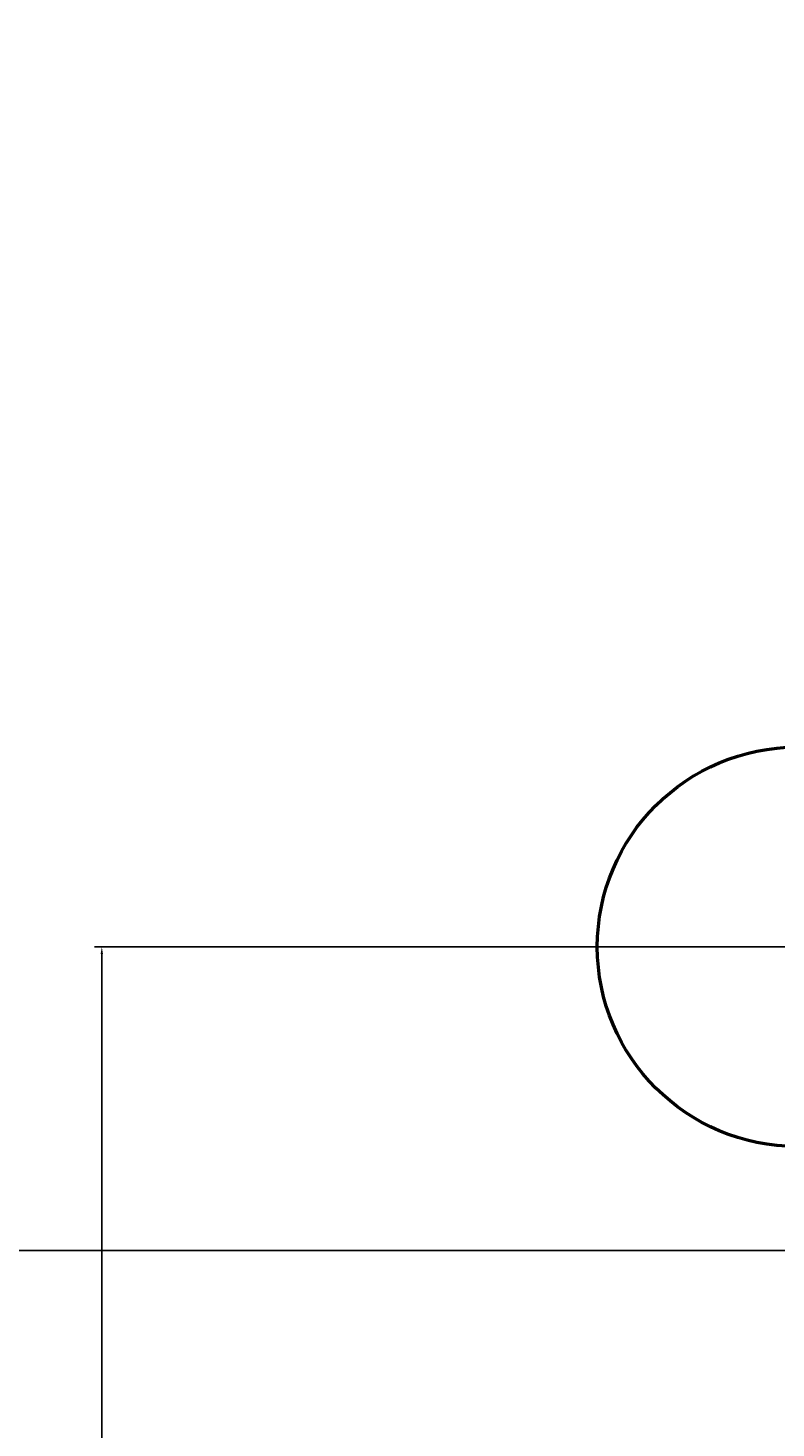
# Model space of a CAD drawing. Units: inches. Extents: x 457 to 775, y 319 to 541.
# Tile 3 of 12: x 536 to 554, y 350 to 385. Entities that reach past the tile are written whole.
import ezdxf

# ---------------------------------------------------------------- set-up
doc = ezdxf.new("R2010")
doc.units = ezdxf.units.IN
doc.header["$MEASUREMENT"] = 0
doc.layers.add('M-DIMS', color=2, linetype='Continuous', lineweight=18)
doc.layers.add('M-OUTL', color=7, linetype='Continuous', lineweight=50)
doc.styles.get("Standard").update_dxf_attribs({"font": 'arial.ttf'})
doc.dimstyles.get("Standard").update_dxf_attribs({"dimtxt": 0.18, "dimasz": 0.18, "dimexe": 0.18, "dimexo": 0.0625, "dimgap": 0.09, "dimtad": 0, "dimtih": 1, "dimtoh": 1, "dimdec": 4, "dimzin": 0, "dimdsep": 46, "dimtxsty": 'Standard', "dimcen": 0.09, "dimadec": 0, "dimazin": 0, "dimtfac": 1, "dimtdec": 4, "dimtofl": 0, "dimtmove": 0, "dimatfit": 3, "dimfxl": 1, "dimtolj": 1, "dimtzin": 0, "dimarcsym": 0})

# ---------------------------------------------------------------- blocks, each defined once
blk = doc.blocks.new('MOUNT-HOLE-D10')
blk.add_circle((5, 5), 5)
blk = doc.blocks.new('*D2')
at = {"layer": 'Defpoints', "color": 0, "transparency": 16777216}
for p in [(756.931, 375.696), (474.306, 336.696), (756.931, 319.296)]:
    blk.add_point(p, dxfattribs=at)
at = {"layer": 'M-DIMS', "color": 0, "lineweight": -2, "transparency": 16777216}
for p, q in [((756.931, 375.634), (756.931, 319.116)), ((474.306, 336.634), (474.306, 319.116)), ((474.486, 319.296), (615.223, 319.296)), ((756.751, 319.296), (616.014, 319.296))]:
    blk.add_line(p, q, dxfattribs=at)
at = {"layer": 'M-DIMS', "color": 0, "transparency": 16777216}
for points in [[(474.486, 319.326), (474.486, 319.266), (474.306, 319.296)], [(756.751, 319.326), (756.751, 319.266), (756.931, 319.296)]]:
    blk.add_solid(points, dxfattribs=at)
at = {"layer": 'M-DIMS', "color": 0, "transparency": 16777216, "insert": (615.619, 319.296), "char_height": 0.18, "attachment_point": 5}
blk.add_mtext('\\A1;282.6', dxfattribs=at)
blk = doc.blocks.new('*D3')
at = {"layer": 'Defpoints', "color": 0, "transparency": 16777216}
for p in [(456.906, 523.213), (646.001, 523.213), (474.306, 336.696)]:
    blk.add_point(p, dxfattribs=at)
at = {"layer": 'M-DIMS', "color": 0, "lineweight": -2, "transparency": 16777216}
for p, q in [((645.939, 523.213), (456.726, 523.213)), ((456.906, 523.033), (456.906, 430.136)), ((456.906, 336.876), (456.906, 429.773)), ((474.244, 336.696), (456.726, 336.696))]:
    blk.add_line(p, q, dxfattribs=at)
at = {"layer": 'M-DIMS', "color": 0, "transparency": 16777216}
for points in [[(456.876, 523.033), (456.936, 523.033), (456.906, 523.213)], [(456.876, 336.876), (456.936, 336.876), (456.906, 336.696)]]:
    blk.add_solid(points, dxfattribs=at)
at = {"layer": 'M-DIMS', "color": 0, "transparency": 16777216, "insert": (456.906, 429.954), "char_height": 0.18, "attachment_point": 5}
blk.add_mtext('\\A1;186.5', dxfattribs=at)
blk = doc.blocks.new('*D6')
at = {"layer": 'Defpoints', "color": 0, "transparency": 16777216}
for p in [(554.931, 354.096), (474.306, 336.696), (554.931, 336.696)]:
    blk.add_point(p, dxfattribs=at)
at = {"layer": 'M-DIMS', "color": 0, "lineweight": -2, "transparency": 16777216}
for p, q in [((474.306, 336.759), (474.306, 354.276)), ((474.486, 354.096), (514.226, 354.096)), ((554.751, 354.096), (515.011, 354.096)), ((554.931, 336.759), (554.931, 354.276))]:
    blk.add_line(p, q, dxfattribs=at)
at = {"layer": 'M-DIMS', "color": 0, "transparency": 16777216}
for points in [[(474.486, 354.126), (474.486, 354.066), (474.306, 354.096)], [(554.751, 354.126), (554.751, 354.066), (554.931, 354.096)]]:
    blk.add_solid(points, dxfattribs=at)
at = {"layer": 'M-DIMS', "color": 0, "transparency": 16777216, "insert": (514.619, 354.096), "char_height": 0.18, "attachment_point": 5}
blk.add_mtext('\\A1;80.62', dxfattribs=at)
blk = doc.blocks.new('*D7')
at = {"layer": 'Defpoints', "color": 0, "transparency": 16777216}
for p in [(537.531, 361.696), (554.931, 361.696), (554.931, 336.696)]:
    blk.add_point(p, dxfattribs=at)
at = {"layer": 'M-DIMS', "color": 0, "lineweight": -2, "transparency": 16777216}
for p, q in [((554.869, 361.696), (537.351, 361.696)), ((537.531, 361.516), (537.531, 349.378)), ((537.531, 336.876), (537.531, 349.014)), ((554.869, 336.696), (537.351, 336.696))]:
    blk.add_line(p, q, dxfattribs=at)
at = {"layer": 'M-DIMS', "color": 0, "transparency": 16777216}
for points in [[(537.501, 361.516), (537.561, 361.516), (537.531, 361.696)], [(537.501, 336.876), (537.561, 336.876), (537.531, 336.696)]]:
    blk.add_solid(points, dxfattribs=at)
at = {"layer": 'M-DIMS', "color": 0, "transparency": 16777216, "insert": (537.531, 349.196), "char_height": 0.18, "attachment_point": 5}
blk.add_mtext('\\A1;25', dxfattribs=at)
blk = doc.blocks.new('*D16')
at = {"layer": 'Defpoints', "color": 0, "transparency": 16777216}
for p in [(554.931, 540.613), (514.502, 430.729), (554.931, 361.696)]:
    blk.add_point(p, dxfattribs=at)
at = {"layer": 'M-DIMS', "color": 0, "lineweight": -2, "transparency": 16777216}
for p, q in [((514.502, 430.791), (514.502, 540.793)), ((554.931, 361.759), (554.931, 540.793)), ((514.682, 540.613), (534.319, 540.613)), ((554.751, 540.613), (535.114, 540.613))]:
    blk.add_line(p, q, dxfattribs=at)
at = {"layer": 'M-DIMS', "color": 0, "transparency": 16777216}
for points in [[(514.682, 540.643), (514.682, 540.583), (514.502, 540.613)], [(554.751, 540.643), (554.751, 540.583), (554.931, 540.613)]]:
    blk.add_solid(points, dxfattribs=at)
at = {"layer": 'M-DIMS', "color": 0, "transparency": 16777216, "insert": (534.716, 540.613), "char_height": 0.18, "attachment_point": 5}
blk.add_mtext('\\A1;40.43', dxfattribs=at)

msp = doc.modelspace()

# ---------------------------------------------------------------- block references
at = {"layer": 'M-OUTL'}
msp.add_blockref('MOUNT-HOLE-D10', (549.931, 356.696), dxfattribs=at)

# ---------------------------------------------------------------- dimensions: what is measured, and where the dimension line sits
at = {"layer": 'M-DIMS'}
for base, p1, p2, override, picture, middle in [((554.931, 540.613), (514.502, 430.729), (554.931, 361.696), {"dimdec": 2, "dimlfac": 1, "dimrnd": 0, "dimzin": 0, "dimdsep": 46, "dimlunit": 2}, '*D16', (534.716, 540.613)), ((756.931, 319.296), (474.306, 336.696), (756.931, 375.696), {"dimdec": 1, "dimlfac": 1, "dimrnd": 0, "dimzin": 0, "dimdsep": 46, "dimlunit": 2}, '*D2', (615.619, 319.296)), ((554.931, 354.096), (474.3061, 336.696), (554.931, 336.696), {"dimdec": 2, "dimlfac": 1, "dimrnd": 0, "dimzin": 0, "dimdsep": 46, "dimlunit": 2}, '*D6', (514.6186, 354.096))]:
    dim = msp.add_linear_dim(base=base, p1=p1, p2=p2, dimstyle='Standard', override=override, dxfattribs=at)
    dim.commit()
    dim.dimension.update_dxf_attribs({"geometry": picture, "text_midpoint": middle})
for base, p1, p2, override, picture, middle in [((456.906, 523.213), (474.306, 336.696), (646.001, 523.213), {"dimdec": 1, "dimlfac": 1, "dimrnd": 0, "dimzin": 0, "dimdsep": 46, "dimlunit": 2}, '*D3', (456.906, 429.954)), ((537.531, 361.696), (554.931, 336.696), (554.931, 361.696), {"dimdec": 0, "dimlfac": 1, "dimrnd": 0, "dimzin": 0, "dimdsep": 46, "dimlunit": 2}, '*D7', (537.531, 349.196))]:
    dim = msp.add_linear_dim(base=base, p1=p1, p2=p2, angle=90, dimstyle='Standard', override=override, dxfattribs=at)
    dim.commit()
    dim.dimension.update_dxf_attribs({"geometry": picture, "text_midpoint": middle})

doc.saveas('drawing.dxf')
